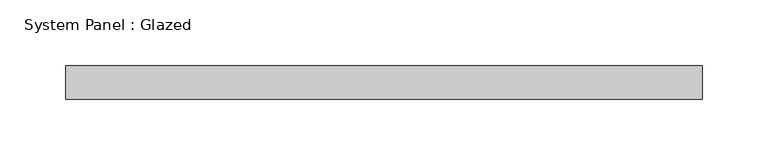
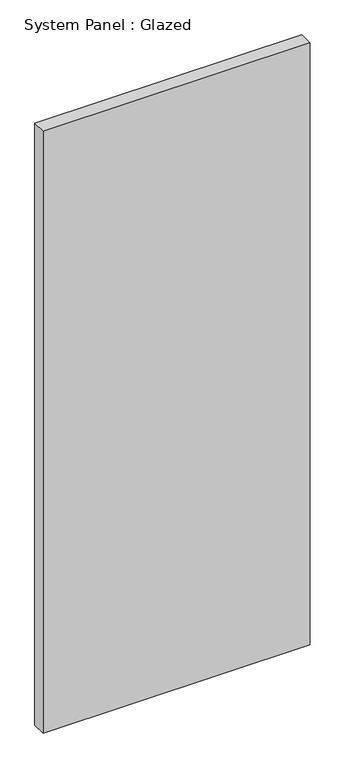
"""IFC4 building model written with IfcOpenShell, lengths in millimetres: plate geometry, System Panel : Glazed."""

from ifc_helpers import new_model, si_unit, origin, origin_with_axes, place, context, project, spatial, polyline, outline, extrude, source, transform, mapped, element, save


def system_panel_glazed_82984963(model_context):
    return source(origin(), model_context, "Body", "SweptSolid", [
        extrude(outline(polyline([(241.3, -44.45), (-241.3, -44.45), (-241.3, -19.05), (241.3, -19.05), (241.3, -44.45)])), origin_with_axes(), (0.0, 0.0, 1.0), 1149.35),
    ])


if __name__ == "__main__":
    model = new_model("IFC4")
    model_context = context("Model", 3, world=origin())
    ifc_project = project(units=[si_unit("LENGTHUNIT", "METRE", prefix="MILLI")], contexts=[model_context])
    site = spatial("IfcSite", under=ifc_project)
    building = spatial("IfcBuilding", under=site)
    placement = place(None, origin())
    system_panel_glazed_shape = system_panel_glazed_82984963(model_context)
    element("IfcPlate", 1, ObjectType="System Panel : Glazed", at=placement, inside=building, context=model_context, shape_type="MappedRepresentation", body=[
        mapped(system_panel_glazed_shape, transform((0.0, 0.0, 0.0), x_axis=(1.0, 0.0, 0.0), y_axis=(0.0, 1.0, 0.0), z_axis=(0.0, 0.0, 1.0))),
    ])
    save(model, "model.ifc")

# Revit data of these elements
# Type "System Panel : Glazed"
#   Construction Type Id = "GSP4R"
#   Analytic Construction = "1/8 in Pilkington single glazing"
#   Visual Light Transmittance = 0.9
#   Solar Heat Gain Coefficient = 0.86
#   Heat Transfer Coefficient (U) = 1.18115 BTU/(h·ft²·°F)
#   Define Thermal Properties by = 1
# Element 1 (IfcPlate, "System Panel : Glazed")
#   Materials on its faces: "Glass"
# Materials
#   "Glass": class "Glass", colour RGB 0 128 192, transparency 0.75, Description = "Soda Lime Glass", Cost = 0
